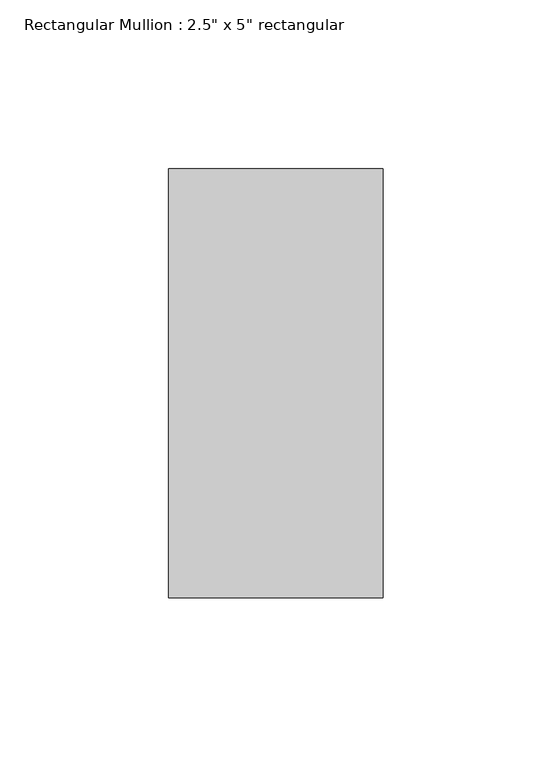
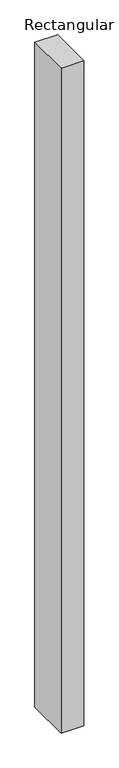
"""IFC4 building model written with IfcOpenShell, lengths in millimetres: member geometry."""

from ifc_helpers import new_model, si_unit, frame, origin, place, context, project, spatial, polyline, outline, extrude, source, transform, mapped, element, save


def member_bbdb212f(model_context):
    return source(origin(), model_context, "Body", "SweptSolid", [
        extrude(outline(polyline([(31.75, 63.5), (31.75, -63.5), (-31.75, -63.5), (-31.75, 63.5), (31.75, 63.5)])), frame((0.0, 0.0, -1970.7905078), z_axis=(0.0, 0.0, 1.0), x_axis=(1.0, 0.0, 0.0)), (0.0, 0.0, 1.0), 1970.7905078),
    ])


if __name__ == "__main__":
    model = new_model("IFC4")
    model_context = context("Model", 3, world=origin())
    ifc_project = project(units=[si_unit("LENGTHUNIT", "METRE", prefix="MILLI")], contexts=[model_context])
    site = spatial("IfcSite", under=ifc_project)
    building = spatial("IfcBuilding", under=site)
    placement = place(None, origin())
    member_shape = member_bbdb212f(model_context)
    element("IfcMember", 1, ObjectType="Rectangular Mullion : 2.5\" x 5\" rectangular", at=placement, inside=building, context=model_context, shape_type="MappedRepresentation", body=[
        mapped(member_shape, transform((0.0, 0.0, 0.0), x_axis=(1.0, 0.0, 0.0), y_axis=(0.0, 1.0, 0.0), z_axis=(0.0, 0.0, 1.0))),
    ])
    save(model, "model.ifc")

# Revit data of these elements
# Type "Rectangular Mullion : 2.5\" x 5\" rectangular"
#   built-in parameter 1007304 = 0.416667 (stored number, unit not read)
#   built-in parameter 1007301 = 0.104167 (stored number, unit not read)
#   built-in parameter 1007300 = 0.104167 (stored number, unit not read)
# Element 1 (IfcMember, "Rectangular Mullion : 2.5\" x 5\" rectangular")
#   Materials on its faces: "Aluminum"
# Materials
#   "Aluminum": class "Metal", colour RGB 247 247 247, transparency 0, Description = "Aluminum 6061", Cost = 0
